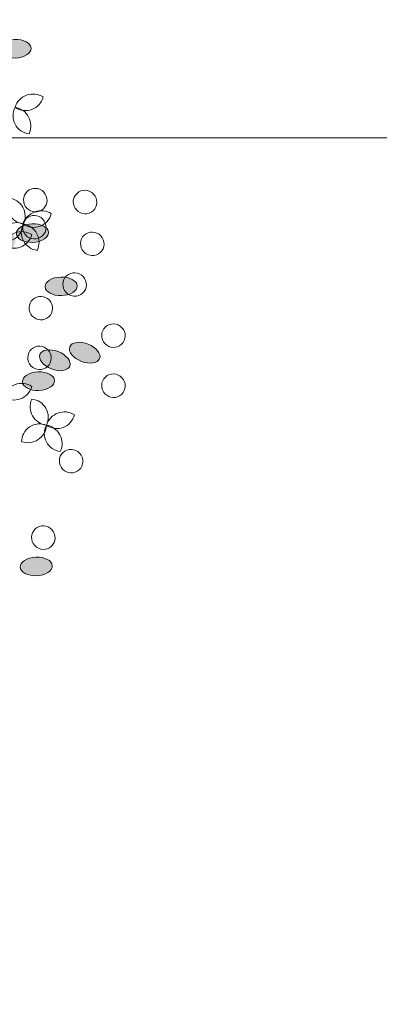
# Model space of a CAD drawing. Units: millimetres. Extents: x 595116 to 630915, y 909473 to 920225.
# Tile 79 of 134: x 629647 to 629661, y 919267 to 919307. Entities that reach past the tile are written whole.
import ezdxf

# ---------------------------------------------------------------- set-up
doc = ezdxf.new("R2010")
doc.units = ezdxf.units.MM
doc.layers.add('Dimension', color=3, linetype='Continuous', lineweight=18)
doc.layers.add('L-PLNT', color=85, linetype='Continuous', lineweight=13)
doc.styles.get("Standard").update_dxf_attribs({"font": 'arial.ttf'})
doc.dimstyles.new('ISO-25', dxfattribs={"dimtxt": 9, "dimasz": 6, "dimexe": 1.25, "dimexo": 0.625, "dimtad": 1, "dimlunit": 4, "dimtxsty": 'Standard', "dimcen": 2.5, "dimadec": 0, "dimazin": 0, "dimtfac": 1, "dimtmove": 0, "dimatfit": 3, "dimfxl": 1, "dimarcsym": 0})

# ---------------------------------------------------------------- blocks, each defined once
blk = doc.blocks.new('A$C77972600')
h = blk.add_hatch(color=256)
edge = h.paths.add_edge_path()
edge.add_ellipse((3.07, 5.828), major_axis=(-0.173, 0.07), ratio=0.578492, start_angle=0, end_angle=360)
edge = h.paths.add_edge_path()
edge.add_ellipse((4.099, 6.003), major_axis=(-0.132, 0.132), ratio=0.578492, start_angle=0, end_angle=360)
edge = h.paths.add_edge_path()
edge.add_ellipse((4.532, 6.768), major_axis=(-0.169, -0.08), ratio=0.578492, start_angle=0, end_angle=360)
edge = h.paths.add_edge_path()
edge.add_ellipse((5.185, 6.87), major_axis=(-0.187, -0.007), ratio=0.578492, start_angle=0, end_angle=360)
edge = h.paths.add_edge_path()
edge.add_ellipse((4.688, 3.446), major_axis=(-0.187, -0.007), ratio=0.578492, start_angle=0, end_angle=360)
edge = h.paths.add_edge_path()
edge.add_ellipse((4.522, 4.237), major_axis=(-0.187, -0.007), ratio=0.578492, start_angle=0, end_angle=360)
edge = h.paths.add_edge_path()
edge.add_ellipse((4.917, 3.995), major_axis=(-0.173, 0.07), ratio=0.578492, start_angle=0, end_angle=360)
edge = h.paths.add_edge_path()
edge.add_ellipse((3.676, 4.999), major_axis=(-0.132, 0.132), ratio=0.578492, start_angle=0, end_angle=360)
edge = h.paths.add_edge_path()
edge.add_ellipse((3.103, 4.678), major_axis=(-0.132, 0.132), ratio=0.578492, start_angle=0, end_angle=360)
edge = h.paths.add_edge_path()
edge.add_ellipse((3.813, 4.558), major_axis=(-0.132, 0.132), ratio=0.578492, start_angle=0, end_angle=360)
edge = h.paths.add_edge_path()
edge.add_ellipse((2.204, 5.633), major_axis=(-0.187, -0.007), ratio=0.578492, start_angle=0, end_angle=360)
edge = h.paths.add_edge_path()
edge.add_ellipse((2.907, 5.654), major_axis=(-0.187, -0.007), ratio=0.578492, start_angle=0, end_angle=360)
edge = h.paths.add_edge_path()
edge.add_ellipse((2.622, 5.434), major_axis=(-0.187, -0.007), ratio=0.578492, start_angle=0, end_angle=360)
edge = h.paths.add_edge_path()
edge.add_ellipse((2.12, 4.017), major_axis=(-0.173, 0.07), ratio=0.578492, start_angle=0, end_angle=360)
edge = h.paths.add_edge_path()
edge.add_ellipse((4.149, 5.591), major_axis=(-0.169, -0.08), ratio=0.578492, start_angle=0, end_angle=360)
edge = h.paths.add_edge_path()
edge.add_ellipse((1.957, 3.173), major_axis=(-0.187, -0.007), ratio=0.578492, start_angle=0, end_angle=360)
edge = h.paths.add_edge_path()
edge.add_ellipse((1.589, 3.291), major_axis=(-0.169, -0.08), ratio=0.578492, start_angle=0, end_angle=360)
edge = h.paths.add_edge_path()
edge.add_ellipse((1.045, 3.081), major_axis=(-0.187, -0.007), ratio=0.578492, start_angle=0, end_angle=360)
edge = h.paths.add_edge_path()
edge.add_ellipse((1.21, 3.774), major_axis=(-0.169, -0.08), ratio=0.578492, start_angle=0, end_angle=360)
edge = h.paths.add_edge_path()
edge.add_ellipse((1.672, 3.755), major_axis=(-0.169, -0.08), ratio=0.578492, start_angle=0, end_angle=360)
edge = h.paths.add_edge_path()
edge.add_ellipse((0.772, 4.473), major_axis=(-0.173, 0.07), ratio=0.578492, start_angle=0, end_angle=360)
edge = h.paths.add_edge_path()
edge.add_ellipse((0.833, 5.292), major_axis=(-0.132, 0.132), ratio=0.578492, start_angle=0, end_angle=360)
edge = h.paths.add_edge_path()
edge.add_ellipse((1.188, 5.231), major_axis=(-0.132, 0.132), ratio=0.578492, start_angle=0, end_angle=360)
edge = h.paths.add_edge_path()
edge.add_ellipse((5.388, 4.72), major_axis=(-0.187, -0.007), ratio=0.578492, start_angle=0, end_angle=360)
edge = h.paths.add_edge_path()
edge.add_ellipse((3.555, 2.162), major_axis=(-0.187, -0.007), ratio=0.578492, start_angle=0, end_angle=360)
edge = h.paths.add_edge_path()
edge.add_ellipse((3.84, 2.382), major_axis=(-0.187, -0.007), ratio=0.578492, start_angle=0, end_angle=360)
edge = h.paths.add_edge_path()
edge.add_ellipse((4.692, 2.204), major_axis=(-0.173, 0.07), ratio=0.578492, start_angle=0, end_angle=360)
edge = h.paths.add_edge_path()
edge.add_ellipse((4.514, 2.91), major_axis=(-0.173, 0.07), ratio=0.578492, start_angle=0, end_angle=360)
edge = h.paths.add_edge_path()
edge.add_ellipse((4.813, 2.558), major_axis=(-0.173, 0.07), ratio=0.578492, start_angle=0, end_angle=360)
edge = h.paths.add_edge_path()
edge.add_ellipse((3.788, 2.89), major_axis=(-0.173, 0.07), ratio=0.578492, start_angle=0, end_angle=360)
h = blk.add_hatch(color=256)
edge = h.paths.add_edge_path()
edge.add_ellipse((3.24, 1.699), major_axis=(-0.167, -0.084), ratio=0.578492, start_angle=0, end_angle=360, ccw=False)
edge = h.paths.add_edge_path()
edge.add_ellipse((4.28, 1.608), major_axis=(-0.121, -0.142), ratio=0.578492, start_angle=0, end_angle=360, ccw=False)
edge = h.paths.add_edge_path()
edge.add_ellipse((4.774, 0.881), major_axis=(-0.175, 0.066), ratio=0.578492, start_angle=0, end_angle=360, ccw=False)
edge = h.paths.add_edge_path()
edge.add_ellipse((5.433, 0.833), major_axis=(-0.187, -0.008), ratio=0.578492, start_angle=0, end_angle=360, ccw=False)
edge = h.paths.add_edge_path()
edge.add_ellipse((4.657, 4.205), major_axis=(-0.187, -0.008), ratio=0.578492, start_angle=0, end_angle=360, ccw=False)
edge = h.paths.add_edge_path()
edge.add_ellipse((4.556, 3.403), major_axis=(-0.187, -0.008), ratio=0.578492, start_angle=0, end_angle=360, ccw=False)
edge = h.paths.add_edge_path()
edge.add_ellipse((4.93, 3.677), major_axis=(-0.167, -0.084), ratio=0.578492, start_angle=0, end_angle=360, ccw=False)
edge = h.paths.add_edge_path()
edge.add_ellipse((3.776, 2.574), major_axis=(-0.121, -0.142), ratio=0.578492, start_angle=0, end_angle=360, ccw=False)
edge = h.paths.add_edge_path()
edge.add_ellipse((3.179, 2.847), major_axis=(-0.121, -0.142), ratio=0.578492, start_angle=0, end_angle=360, ccw=False)
edge = h.paths.add_edge_path()
edge.add_ellipse((3.876, 3.025), major_axis=(-0.121, -0.142), ratio=0.578492, start_angle=0, end_angle=360, ccw=False)
edge = h.paths.add_edge_path()
edge.add_ellipse((2.361, 1.822), major_axis=(-0.187, -0.008), ratio=0.578492, start_angle=0, end_angle=360, ccw=False)
edge = h.paths.add_edge_path()
edge.add_ellipse((3.063, 1.858), major_axis=(-0.187, -0.008), ratio=0.578492, start_angle=0, end_angle=360, ccw=False)
edge = h.paths.add_edge_path()
edge.add_ellipse((2.761, 2.054), major_axis=(-0.187, -0.008), ratio=0.578492, start_angle=0, end_angle=360, ccw=False)
edge = h.paths.add_edge_path()
edge.add_ellipse((2.144, 3.425), major_axis=(-0.167, -0.084), ratio=0.578492, start_angle=0, end_angle=360, ccw=False)
edge = h.paths.add_edge_path()
edge.add_ellipse((4.296, 2.022), major_axis=(-0.175, 0.066), ratio=0.578492, start_angle=0, end_angle=360, ccw=False)
edge = h.paths.add_edge_path()
edge.add_ellipse((1.913, 4.253), major_axis=(-0.187, -0.008), ratio=0.578492, start_angle=0, end_angle=360, ccw=False)
edge = h.paths.add_edge_path()
edge.add_ellipse((1.556, 4.105), major_axis=(-0.175, 0.066), ratio=0.578492, start_angle=0, end_angle=360, ccw=False)
edge = h.paths.add_edge_path()
edge.add_ellipse((0.996, 4.269), major_axis=(-0.187, -0.008), ratio=0.578492, start_angle=0, end_angle=360, ccw=False)
edge = h.paths.add_edge_path()
edge.add_ellipse((1.218, 3.593), major_axis=(-0.175, 0.066), ratio=0.578492, start_angle=0, end_angle=360, ccw=False)
edge = h.paths.add_edge_path()
edge.add_ellipse((1.676, 3.649), major_axis=(-0.175, 0.066), ratio=0.578492, start_angle=0, end_angle=360, ccw=False)
edge = h.paths.add_edge_path()
edge.add_ellipse((0.838, 2.86), major_axis=(-0.167, -0.084), ratio=0.578492, start_angle=0, end_angle=360, ccw=False)
edge = h.paths.add_edge_path()
edge.add_ellipse((0.966, 2.049), major_axis=(-0.121, -0.142), ratio=0.578492, start_angle=0, end_angle=360, ccw=False)
edge = h.paths.add_edge_path()
edge.add_ellipse((1.315, 2.138), major_axis=(-0.121, -0.142), ratio=0.578492, start_angle=0, end_angle=360, ccw=False)
edge = h.paths.add_edge_path()
edge.add_ellipse((5.459, 2.993), major_axis=(-0.187, -0.008), ratio=0.578492, start_angle=0, end_angle=360, ccw=False)
edge = h.paths.add_edge_path()
edge.add_ellipse((3.422, 5.392), major_axis=(-0.187, -0.008), ratio=0.578492, start_angle=0, end_angle=360, ccw=False)
edge = h.paths.add_edge_path()
edge.add_ellipse((3.725, 5.196), major_axis=(-0.187, -0.008), ratio=0.578492, start_angle=0, end_angle=360, ccw=False)
edge = h.paths.add_edge_path()
edge.add_ellipse((4.559, 5.443), major_axis=(-0.167, -0.084), ratio=0.578492, start_angle=0, end_angle=360, ccw=False)
edge = h.paths.add_edge_path()
edge.add_ellipse((4.439, 4.725), major_axis=(-0.167, -0.084), ratio=0.578492, start_angle=0, end_angle=360, ccw=False)
edge = h.paths.add_edge_path()
edge.add_ellipse((4.709, 5.101), major_axis=(-0.167, -0.084), ratio=0.578492, start_angle=0, end_angle=360, ccw=False)
edge = h.paths.add_edge_path()
edge.add_ellipse((3.714, 4.685), major_axis=(-0.167, -0.084), ratio=0.578492, start_angle=0, end_angle=360, ccw=False)
h = blk.add_hatch(color=256)
edge = h.paths.add_edge_path()
edge.add_ellipse((4.165, 1.933), major_axis=(0.187, 0.006), ratio=0.578492, start_angle=0, end_angle=360)
edge = h.paths.add_edge_path()
edge.add_ellipse((3.294, 1.359), major_axis=(0.174, -0.068), ratio=0.578492, start_angle=0, end_angle=360)
edge = h.paths.add_edge_path()
edge.add_ellipse((3.206, 0.484), major_axis=(0.122, 0.141), ratio=0.578492, start_angle=0, end_angle=360)
edge = h.paths.add_edge_path()
edge.add_ellipse((2.65, 0.127), major_axis=(0.168, 0.082), ratio=0.578492, start_angle=0, end_angle=360)
edge = h.paths.add_edge_path()
edge.add_ellipse((1.725, 3.461), major_axis=(0.168, 0.082), ratio=0.578492, start_angle=0, end_angle=360)
edge = h.paths.add_edge_path()
edge.add_ellipse((2.196, 2.805), major_axis=(0.168, 0.082), ratio=0.578492, start_angle=0, end_angle=360)
edge = h.paths.add_edge_path()
edge.add_ellipse((1.737, 2.867), major_axis=(0.187, 0.006), ratio=0.578492, start_angle=0, end_angle=360)
edge = h.paths.add_edge_path()
edge.add_ellipse((3.277, 2.448), major_axis=(0.174, -0.068), ratio=0.578492, start_angle=0, end_angle=360)
edge = h.paths.add_edge_path()
edge.add_ellipse((3.672, 2.972), major_axis=(0.174, -0.068), ratio=0.578492, start_angle=0, end_angle=360)
edge = h.paths.add_edge_path()
edge.add_ellipse((2.974, 2.796), major_axis=(0.174, -0.068), ratio=0.578492, start_angle=0, end_angle=360)
edge = h.paths.add_edge_path()
edge.add_ellipse((4.88, 2.46), major_axis=(0.168, 0.082), ratio=0.578492, start_angle=0, end_angle=360)
edge = h.paths.add_edge_path()
edge.add_ellipse((4.245, 2.158), major_axis=(0.168, 0.082), ratio=0.578492, start_angle=0, end_angle=360)
edge = h.paths.add_edge_path()
edge.add_ellipse((4.418, 2.474), major_axis=(0.168, 0.082), ratio=0.578492, start_angle=0, end_angle=360)
edge = h.paths.add_edge_path()
edge.add_ellipse((4.307, 3.973), major_axis=(0.187, 0.006), ratio=0.578492, start_angle=0, end_angle=360)
edge = h.paths.add_edge_path()
edge.add_ellipse((3.083, 1.715), major_axis=(0.122, 0.141), ratio=0.578492, start_angle=0, end_angle=360)
edge = h.paths.add_edge_path()
edge.add_ellipse((4.115, 4.811), major_axis=(0.168, 0.082), ratio=0.578492, start_angle=0, end_angle=360)
edge = h.paths.add_edge_path()
edge.add_ellipse((4.5, 4.852), major_axis=(0.122, 0.141), ratio=0.578492, start_angle=0, end_angle=360)
edge = h.paths.add_edge_path()
edge.add_ellipse((4.913, 5.263), major_axis=(0.168, 0.082), ratio=0.578492, start_angle=0, end_angle=360)
edge = h.paths.add_edge_path()
edge.add_ellipse((5.041, 4.562), major_axis=(0.122, 0.141), ratio=0.578492, start_angle=0, end_angle=360)
edge = h.paths.add_edge_path()
edge.add_ellipse((4.61, 4.393), major_axis=(0.122, 0.141), ratio=0.578492, start_angle=0, end_angle=360)
edge = h.paths.add_edge_path()
edge.add_ellipse((5.723, 4.099), major_axis=(0.187, 0.006), ratio=0.578492, start_angle=0, end_angle=360)
edge = h.paths.add_edge_path()
edge.add_ellipse((5.998, 3.325), major_axis=(0.174, -0.068), ratio=0.578492, start_angle=0, end_angle=360)
edge = h.paths.add_edge_path()
edge.add_ellipse((5.649, 3.237), major_axis=(0.174, -0.068), ratio=0.578492, start_angle=0, end_angle=360)
edge = h.paths.add_edge_path()
edge.add_ellipse((1.598, 2.014), major_axis=(0.168, 0.082), ratio=0.578492, start_angle=0, end_angle=360)
edge = h.paths.add_edge_path()
edge.add_ellipse((2.245, 5.093), major_axis=(0.168, 0.082), ratio=0.578492, start_angle=0, end_angle=360)
edge = h.paths.add_edge_path()
edge.add_ellipse((2.073, 4.777), major_axis=(0.168, 0.082), ratio=0.578492, start_angle=0, end_angle=360)
edge = h.paths.add_edge_path()
edge.add_ellipse((1.222, 4.597), major_axis=(0.187, 0.006), ratio=0.578492, start_angle=0, end_angle=360)
edge = h.paths.add_edge_path()
edge.add_ellipse((1.669, 4.023), major_axis=(0.187, 0.006), ratio=0.578492, start_angle=0, end_angle=360)
edge = h.paths.add_edge_path()
edge.add_ellipse((1.253, 4.224), major_axis=(0.187, 0.006), ratio=0.578492, start_angle=0, end_angle=360)
edge = h.paths.add_edge_path()
edge.add_ellipse((2.326, 4.333), major_axis=(0.187, 0.006), ratio=0.578492, start_angle=0, end_angle=360)
for centre, radius, start, end in [((5.395, 6.123), 0.219, 57.5868, 162.9238), ((5.308, 6.359), 0.211, 234.6671, 345.8435), ((5.373, 6.088), 0.211, 152.1384, 263.3149), ((5.15, 5.971), 0.219, 335.0581, 80.3951), ((5.312, 5.043), 0.219, 156.8071, 262.1441), ((5.093, 4.919), 0.211, 333.8874, 85.0638), ((5.491, 4.762), 0.219, 57.5868, 162.9238), ((5.404, 4.998), 0.211, 234.6671, 345.8435), ((5.204, 4.631), 0.211, 68.147, 179.3234), ((5.064, 4.84), 0.219, 251.0667, 356.4037), ((5.469, 4.728), 0.211, 152.1384, 263.3149), ((5.246, 4.611), 0.219, 335.0581, 80.3951), ((5.263, 4.518), 0.219, 57.5868, 162.9238), ((5.175, 4.754), 0.211, 234.6671, 345.8435), ((5.263, 2.748), 0.219, 57.5868, 162.9238), ((5.175, 2.984), 0.211, 234.6671, 345.8435), ((5.581, 2.696), 0.219, 156.8071, 262.1441), ((5.362, 2.573), 0.211, 333.8874, 85.0638), ((5.761, 2.416), 0.219, 57.5868, 162.9238), ((5.673, 2.652), 0.211, 234.6671, 345.8435), ((5.473, 2.284), 0.211, 68.147, 179.3234), ((5.334, 2.494), 0.219, 251.0667, 356.4037), ((5.738, 2.382), 0.211, 152.1384, 263.3149), ((5.515, 2.265), 0.219, 335.0581, 80.3951)]:
    blk.add_arc(centre, radius, start, end)
for centre, major_axis, start_param, end_param in [((5.185, 6.87), (-0.187, -0.007), 1.570796326839852, 7.853981634019438), ((5.388, 4.72), (-0.187, -0.007), 1.570796326819928, 7.853981633999514), ((5.723, 4.099), (-0.187, -0.006), 4.712389, 10.995574), ((5.998, 3.325), (-0.174, 0.068), 3.141593, 9.424778), ((5.649, 3.237), (-0.174, 0.068), 3.141593, 9.424778)]:
    blk.add_ellipse(centre, major_axis=major_axis, ratio=0.578492, start_param=start_param, end_param=end_param)
for centre in [(5.422, 5.105), (6.002, 5.082), (5.41, 4.789), (6.086, 4.595), (5.88, 4.12), (5.486, 3.845), (6.333, 3.524), (5.471, 3.265), (6.333, 2.94), (5.839, 2.06), (5.515, 1.169)]:
    blk.add_ellipse(centre, major_axis=(-0.094, 0.101), ratio=0.985729)
at = {"extrusion": (0, 0, -1)}
for centre in [(5.459, 2.993), (5.433, 0.833)]:
    blk.add_ellipse(centre, major_axis=(-0.187, -0.008), ratio=0.578492, start_param=3.141593, end_param=9.424778, dxfattribs=at)
blk = doc.blocks.new('*D211')
at = {"layer": 'Defpoints', "color": 0, "transparency": 16777216}
for p in [(629535.386, 919258.662), (629586.227, 919258.662), (629586.227, 919250.943)]:
    blk.add_point(p, dxfattribs=at)
at = {"layer": 'Dimension', "color": 0, "lineweight": -2, "transparency": 16777216}
for p, q in [((629535.386, 919258.037), (629535.386, 919249.693)), ((629586.227, 919258.037), (629586.227, 919249.693)), ((629541.386, 919250.943), (629580.227, 919250.943)), ((629586.227, 919250.943), (629648.699, 919250.943))]:
    blk.add_line(p, q, dxfattribs=at)
at = {"layer": 'Dimension', "color": 0, "transparency": 16777216}
for points in [[(629541.386, 919251.943), (629541.386, 919249.943), (629535.386, 919250.943)], [(629580.227, 919251.943), (629580.227, 919249.943), (629586.227, 919250.943)]]:
    blk.add_solid(points, dxfattribs=at)
at = {"layer": 'Dimension', "color": 0, "transparency": 16777216, "insert": (629620.463, 919256.167), "char_height": 9, "attachment_point": 5}
blk.add_mtext('4\'-3" TYP.', dxfattribs=at)
blk = doc.blocks.new('*D216')
at = {"layer": 'Defpoints', "color": 0, "transparency": 16777216}
for p in [(629743.541, 919411.928), (629505.041, 919411.828), (629743.541, 918832.378)]:
    blk.add_point(p, dxfattribs=at)
at = {"layer": 'Dimension', "color": 0, "lineweight": -2, "transparency": 16777216}
for p, q in [((629505.041, 919411.203), (629505.041, 918831.128)), ((629743.541, 919411.303), (629743.541, 918831.128)), ((629511.041, 918832.378), (629737.541, 918832.378))]:
    blk.add_line(p, q, dxfattribs=at)
at = {"layer": 'Dimension', "color": 0, "transparency": 16777216}
for points in [[(629511.041, 918833.378), (629511.041, 918831.378), (629505.041, 918832.378)], [(629737.541, 918833.378), (629737.541, 918831.378), (629743.541, 918832.378)]]:
    blk.add_solid(points, dxfattribs=at)
at = {"layer": 'Dimension', "color": 0, "transparency": 16777216, "insert": (629624.291, 918837.656), "char_height": 9, "attachment_point": 5}
blk.add_mtext('19\'-10 1/2"', dxfattribs=at)
blk = doc.blocks.new('*D220')
at = {"layer": 'Defpoints', "color": 0, "transparency": 16777216}
for p in [(629824.951, 920160.756), (629511.274, 919302.009), (629824.951, 919302.009)]:
    blk.add_point(p, dxfattribs=at)
at = {"layer": 'Dimension', "color": 0, "lineweight": -2, "transparency": 16777216}
for p, q in [((629511.274, 919302.634), (629511.274, 920162.006)), ((629824.951, 919302.634), (629824.951, 920162.006)), ((629517.274, 920160.756), (629818.951, 920160.756))]:
    blk.add_line(p, q, dxfattribs=at)
at = {"layer": 'Dimension', "color": 0, "transparency": 16777216}
for points in [[(629517.274, 920161.756), (629517.274, 920159.756), (629511.274, 920160.756)], [(629818.951, 920161.756), (629818.951, 920159.756), (629824.951, 920160.756)]]:
    blk.add_solid(points, dxfattribs=at)
at = {"layer": 'Dimension', "color": 0, "transparency": 16777216, "insert": (629668.113, 920166.035), "char_height": 9, "attachment_point": 5}
blk.add_mtext('26\'-1 1/2"', dxfattribs=at)

msp = doc.modelspace()

# ---------------------------------------------------------------- linework, layer by layer
at = {"layer": 'L-PLNT'}
msp.add_line((629824.951, 919302.009), (629511.274, 919302.009), dxfattribs=at)

# ---------------------------------------------------------------- block references
at = {"layer": 'L-PLNT', "xscale": 3.512546757812034, "yscale": 3.512546757812034, "zscale": 3.512546757812034}
msp.add_blockref('A$C77972600', (629628.32, 919281.523), dxfattribs=at)

# ---------------------------------------------------------------- dimensions: what is measured, and where the dimension line sits
at = {"layer": 'Dimension'}
for base, p1, p2, picture, middle in [((629824.951, 920160.756), (629511.274, 919302.009), (629824.951, 919302.009), '*D220', (629668.113, 920166.035)), ((629743.541, 918832.378), (629505.041, 919411.828), (629743.541, 919411.928), '*D216', (629624.291, 918837.656))]:
    dim = msp.add_linear_dim(base=base, p1=p1, p2=p2, dimstyle='ISO-25', override={"dimdec": 1, "dimlfac": 1, "dimrnd": 0, "dimzin": 1, "dimdsep": 46, "dimlunit": 4, "dimfrac": 2}, dxfattribs=at)
    dim.commit()
    dim.dimension.update_dxf_attribs({"geometry": picture, "text_midpoint": middle})
dim = msp.add_linear_dim(base=(629586.227, 919250.943), p1=(629535.386, 919258.662), p2=(629586.227, 919258.662), text='<> TYP.', dimstyle='ISO-25', override={"dimdec": 1, "dimlfac": 1, "dimrnd": 0, "dimzin": 1, "dimdsep": 46, "dimlunit": 4, "dimfrac": 2}, dxfattribs=at)
dim.commit()
dim.dimension.update_dxf_attribs({"geometry": '*D211', "text_midpoint": (629620.463, 919256.167)})

doc.saveas('drawing.dxf')
